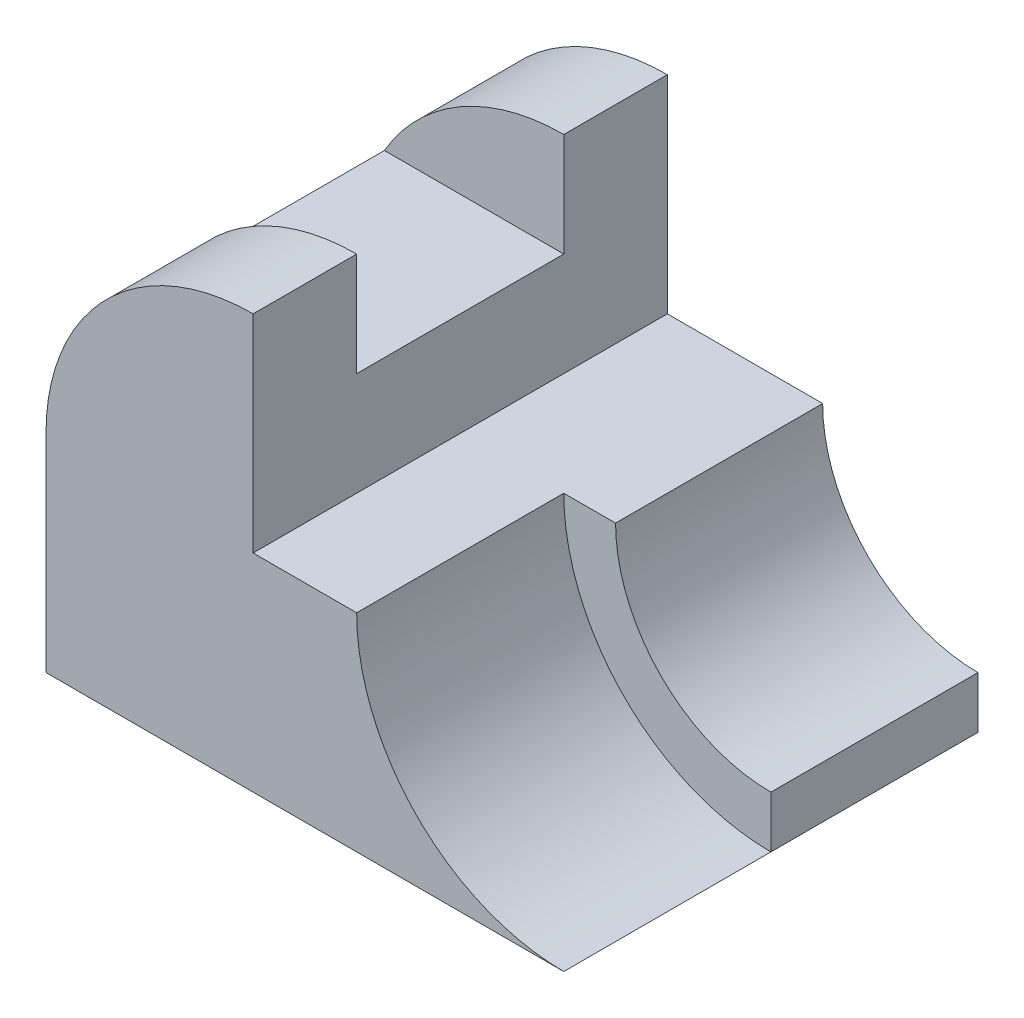
ISO-10303-21;
HEADER;
FILE_DESCRIPTION(('STEP AP214'),'2;1');
FILE_NAME('part.step','',(''),(''),'','','');
FILE_SCHEMA(('AUTOMOTIVE_DESIGN { 1 0 10303 214 1 1 1 1 }'));
ENDSEC;
DATA;
#1=APPLICATION_CONTEXT('core data for automotive mechanical design processes');
#2=APPLICATION_PROTOCOL_DEFINITION('international standard','automotive_design',2000,#1);
#3=PRODUCT_CONTEXT('',#1,'mechanical');
#4=PRODUCT('Part','Part','',(#3));
#5=PRODUCT_RELATED_PRODUCT_CATEGORY('part','',(#4));
#6=PRODUCT_DEFINITION_FORMATION('','',#4);
#7=PRODUCT_DEFINITION_CONTEXT('part definition',#1,'design');
#8=PRODUCT_DEFINITION('design','',#6,#7);
#9=PRODUCT_DEFINITION_SHAPE('','',#8);
#10=(LENGTH_UNIT() NAMED_UNIT(*) SI_UNIT(.MILLI.,.METRE.));
#11=(NAMED_UNIT(*) PLANE_ANGLE_UNIT() SI_UNIT($,.RADIAN.));
#12=(NAMED_UNIT(*) SI_UNIT($,.STERADIAN.) SOLID_ANGLE_UNIT());
#13=UNCERTAINTY_MEASURE_WITH_UNIT(LENGTH_MEASURE(1.E-05),#10,'distance_accuracy_value','');
#14=(GEOMETRIC_REPRESENTATION_CONTEXT(3) GLOBAL_UNCERTAINTY_ASSIGNED_CONTEXT((#13)) GLOBAL_UNIT_ASSIGNED_CONTEXT((#10,
#11,#12)) REPRESENTATION_CONTEXT('',''));
#15=CARTESIAN_POINT('',(0.,0.,0.));
#16=DIRECTION('',(0.,0.,1.));
#17=DIRECTION('',(1.,0.,0.));
#18=AXIS2_PLACEMENT_3D('',#15,#16,#17);
#19=CARTESIAN_POINT('',(50.,20.,-20.));
#20=DIRECTION('',(0.,-1.,0.));
#21=DIRECTION('',(1.,0.,0.));
#22=AXIS2_PLACEMENT_3D('',#19,#20,#21);
#23=PLANE('',#22);
#24=DIRECTION('',(1.,0.,0.));
#25=VECTOR('',#24,1.);
#26=CARTESIAN_POINT('',(50.,20.,-20.));
#27=LINE('',#26,#25);
#28=CARTESIAN_POINT('',(20.,20.,-20.));
#29=VERTEX_POINT('',#28);
#30=CARTESIAN_POINT('',(35.,20.,-20.));
#31=VERTEX_POINT('',#30);
#32=EDGE_CURVE('E173',#29,#31,#27,.T.);
#33=ORIENTED_EDGE('',*,*,#32,.F.);
#34=DIRECTION('',(0.,0.,1.));
#35=VECTOR('',#34,1.);
#36=CARTESIAN_POINT('',(20.,20.,-20.));
#37=LINE('',#36,#35);
#38=CARTESIAN_POINT('',(20.,20.,20.));
#39=VERTEX_POINT('',#38);
#40=EDGE_CURVE('E156',#29,#39,#37,.T.);
#41=ORIENTED_EDGE('',*,*,#40,.T.);
#42=DIRECTION('',(1.,0.,0.));
#43=VECTOR('',#42,1.);
#44=CARTESIAN_POINT('',(20.,20.,20.));
#45=LINE('',#44,#43);
#46=CARTESIAN_POINT('',(30.,20.,20.));
#47=VERTEX_POINT('',#46);
#48=EDGE_CURVE('E220',#39,#47,#45,.T.);
#49=ORIENTED_EDGE('',*,*,#48,.T.);
#50=DIRECTION('',(0.,0.,1.));
#51=VECTOR('',#50,1.);
#52=CARTESIAN_POINT('',(30.,20.,0.));
#53=LINE('',#52,#51);
#54=CARTESIAN_POINT('',(30.,20.,0.));
#55=VERTEX_POINT('',#54);
#56=EDGE_CURVE('E177',#55,#47,#53,.T.);
#57=ORIENTED_EDGE('',*,*,#56,.F.);
#58=DIRECTION('',(-1.,0.,0.));
#59=VECTOR('',#58,1.);
#60=CARTESIAN_POINT('',(30.,20.,0.));
#61=LINE('',#60,#59);
#62=CARTESIAN_POINT('',(35.,20.,0.));
#63=VERTEX_POINT('',#62);
#64=EDGE_CURVE('E185',#63,#55,#61,.T.);
#65=ORIENTED_EDGE('',*,*,#64,.F.);
#66=DIRECTION('',(0.,0.,1.));
#67=VECTOR('',#66,1.);
#68=CARTESIAN_POINT('',(35.,20.,-20.));
#69=LINE('',#68,#67);
#70=EDGE_CURVE('E53',#31,#63,#69,.T.);
#71=ORIENTED_EDGE('',*,*,#70,.F.);
#72=EDGE_LOOP('',(#33,#41,#49,#57,#65,#71));
#73=FACE_BOUND('',#72,.T.);
#74=ADVANCED_FACE('F39',(#73),#23,.F.);
#75=CARTESIAN_POINT('',(20.,43.4081818897871,9.99999999999999));
#76=DIRECTION('',(0.,0.,1.));
#77=DIRECTION('',(0.,-1.,0.));
#78=AXIS2_PLACEMENT_3D('',#75,#76,#77);
#79=PLANE('',#78);
#80=DIRECTION('',(1.,0.,0.));
#81=VECTOR('',#80,1.);
#82=CARTESIAN_POINT('',(19.9999999999999,30.,9.99999999999999));
#83=LINE('',#82,#81);
#84=CARTESIAN_POINT('',(2.67949192431127,30.,10.));
#85=VERTEX_POINT('',#84);
#86=CARTESIAN_POINT('',(19.9999999999999,30.,9.99999999999999));
#87=VERTEX_POINT('',#86);
#88=EDGE_CURVE('E147',#85,#87,#83,.T.);
#89=ORIENTED_EDGE('',*,*,#88,.F.);
#90=CARTESIAN_POINT('',(20.,19.9999999999999,10.));
#91=DIRECTION('',(0.,0.,1.));
#92=DIRECTION('',(0.,-1.,0.));
#93=AXIS2_PLACEMENT_3D('',#90,#91,#92);
#94=CIRCLE('',#93,20.);
#95=CARTESIAN_POINT('',(20.,40.,10.));
#96=VERTEX_POINT('',#95);
#97=EDGE_CURVE('E11',#96,#85,#94,.T.);
#98=ORIENTED_EDGE('',*,*,#97,.F.);
#99=DIRECTION('',(0.,1.,0.));
#100=VECTOR('',#99,1.);
#101=CARTESIAN_POINT('',(20.,43.4081818897871,9.99999999999999));
#102=LINE('',#101,#100);
#103=EDGE_CURVE('E214',#87,#96,#102,.T.);
#104=ORIENTED_EDGE('',*,*,#103,.F.);
#105=EDGE_LOOP('',(#89,#98,#104));
#106=FACE_BOUND('',#105,.T.);
#107=ADVANCED_FACE('F226',(#106),#79,.F.);
#108=CARTESIAN_POINT('',(20.,43.4081818897871,-10.));
#109=DIRECTION('',(0.,0.,-1.));
#110=DIRECTION('',(0.,1.,0.));
#111=AXIS2_PLACEMENT_3D('',#108,#109,#110);
#112=PLANE('',#111);
#113=DIRECTION('',(-1.,0.,0.));
#114=VECTOR('',#113,1.);
#115=CARTESIAN_POINT('',(0.,30.,-10.));
#116=LINE('',#115,#114);
#117=CARTESIAN_POINT('',(20.,30.,-10.));
#118=VERTEX_POINT('',#117);
#119=CARTESIAN_POINT('',(2.67949192431126,30.,-10.));
#120=VERTEX_POINT('',#119);
#121=EDGE_CURVE('E146',#118,#120,#116,.T.);
#122=ORIENTED_EDGE('',*,*,#121,.F.);
#123=DIRECTION('',(0.,-1.,0.));
#124=VECTOR('',#123,1.);
#125=CARTESIAN_POINT('',(20.,43.4081818897871,-10.));
#126=LINE('',#125,#124);
#127=CARTESIAN_POINT('',(20.,40.,-10.));
#128=VERTEX_POINT('',#127);
#129=EDGE_CURVE('E157',#128,#118,#126,.T.);
#130=ORIENTED_EDGE('',*,*,#129,.F.);
#131=CARTESIAN_POINT('',(20.,19.9999999999999,-10.));
#132=DIRECTION('',(0.,0.,-1.));
#133=DIRECTION('',(0.,1.,0.));
#134=AXIS2_PLACEMENT_3D('',#131,#132,#133);
#135=CIRCLE('',#134,20.);
#136=EDGE_CURVE('E50',#120,#128,#135,.T.);
#137=ORIENTED_EDGE('',*,*,#136,.F.);
#138=EDGE_LOOP('',(#122,#130,#137));
#139=FACE_BOUND('',#138,.T.);
#140=ADVANCED_FACE('F158',(#139),#112,.F.);
#141=CARTESIAN_POINT('',(50.,0.,20.));
#142=DIRECTION('',(-1.,0.,0.));
#143=DIRECTION('',(0.,-1.,0.));
#144=AXIS2_PLACEMENT_3D('',#141,#142,#143);
#145=PLANE('',#144);
#146=DIRECTION('',(0.,1.,0.));
#147=VECTOR('',#146,1.);
#148=CARTESIAN_POINT('',(50.,0.,-20.));
#149=LINE('',#148,#147);
#150=CARTESIAN_POINT('',(50.,0.,-20.));
#151=VERTEX_POINT('',#150);
#152=CARTESIAN_POINT('',(50.,5.,-20.));
#153=VERTEX_POINT('',#152);
#154=EDGE_CURVE('E168',#151,#153,#149,.T.);
#155=ORIENTED_EDGE('',*,*,#154,.T.);
#156=DIRECTION('',(0.,0.,1.));
#157=VECTOR('',#156,1.);
#158=CARTESIAN_POINT('',(50.,5.,-20.));
#159=LINE('',#158,#157);
#160=CARTESIAN_POINT('',(50.,5.,0.));
#161=VERTEX_POINT('',#160);
#162=EDGE_CURVE('E187',#153,#161,#159,.T.);
#163=ORIENTED_EDGE('',*,*,#162,.T.);
#164=DIRECTION('',(0.,1.,0.));
#165=VECTOR('',#164,1.);
#166=CARTESIAN_POINT('',(50.,0.,0.));
#167=LINE('',#166,#165);
#168=CARTESIAN_POINT('',(50.,0.,0.));
#169=VERTEX_POINT('',#168);
#170=EDGE_CURVE('E186',#169,#161,#167,.T.);
#171=ORIENTED_EDGE('',*,*,#170,.F.);
#172=DIRECTION('',(0.,0.,-1.));
#173=VECTOR('',#172,1.);
#174=CARTESIAN_POINT('',(50.,0.,20.));
#175=LINE('',#174,#173);
#176=EDGE_CURVE('E164',#169,#151,#175,.T.);
#177=ORIENTED_EDGE('',*,*,#176,.T.);
#178=EDGE_LOOP('',(#155,#163,#171,#177));
#179=FACE_BOUND('',#178,.T.);
#180=ADVANCED_FACE('F245',(#179),#145,.F.);
#181=CARTESIAN_POINT('',(0.,0.,20.));
#182=DIRECTION('',(1.,0.,0.));
#183=DIRECTION('',(0.,1.,0.));
#184=AXIS2_PLACEMENT_3D('',#181,#182,#183);
#185=PLANE('',#184);
#186=DIRECTION('',(0.,-1.,0.));
#187=VECTOR('',#186,1.);
#188=CARTESIAN_POINT('',(0.,0.,20.));
#189=LINE('',#188,#187);
#190=CARTESIAN_POINT('',(0.,20.,20.));
#191=VERTEX_POINT('',#190);
#192=CARTESIAN_POINT('',(0.,0.,20.));
#193=VERTEX_POINT('',#192);
#194=EDGE_CURVE('E64',#191,#193,#189,.T.);
#195=ORIENTED_EDGE('',*,*,#194,.F.);
#196=DIRECTION('',(0.,0.,1.));
#197=VECTOR('',#196,1.);
#198=CARTESIAN_POINT('',(0.,20.,-20.));
#199=LINE('',#198,#197);
#200=CARTESIAN_POINT('',(0.,20.,-20.));
#201=VERTEX_POINT('',#200);
#202=EDGE_CURVE('E198',#201,#191,#199,.T.);
#203=ORIENTED_EDGE('',*,*,#202,.F.);
#204=DIRECTION('',(0.,-1.,0.));
#205=VECTOR('',#204,1.);
#206=CARTESIAN_POINT('',(0.,0.,-20.));
#207=LINE('',#206,#205);
#208=CARTESIAN_POINT('',(0.,0.,-20.));
#209=VERTEX_POINT('',#208);
#210=EDGE_CURVE('E80',#201,#209,#207,.T.);
#211=ORIENTED_EDGE('',*,*,#210,.T.);
#212=DIRECTION('',(0.,0.,-1.));
#213=VECTOR('',#212,1.);
#214=CARTESIAN_POINT('',(0.,0.,20.));
#215=LINE('',#214,#213);
#216=EDGE_CURVE('E159',#193,#209,#215,.T.);
#217=ORIENTED_EDGE('',*,*,#216,.F.);
#218=EDGE_LOOP('',(#195,#203,#211,#217));
#219=FACE_BOUND('',#218,.T.);
#220=ADVANCED_FACE('F41',(#219),#185,.F.);
#221=CARTESIAN_POINT('',(0.,0.,20.));
#222=DIRECTION('',(0.,1.,0.));
#223=DIRECTION('',(0.,0.,1.));
#224=AXIS2_PLACEMENT_3D('',#221,#222,#223);
#225=PLANE('',#224);
#226=DIRECTION('',(1.,0.,0.));
#227=VECTOR('',#226,1.);
#228=CARTESIAN_POINT('',(0.,0.,-20.));
#229=LINE('',#228,#227);
#230=EDGE_CURVE('E169',#209,#151,#229,.T.);
#231=ORIENTED_EDGE('',*,*,#230,.T.);
#232=ORIENTED_EDGE('',*,*,#176,.F.);
#233=CARTESIAN_POINT('',(50.,0.,20.));
#234=VERTEX_POINT('',#233);
#235=EDGE_CURVE('E81',#234,#169,#175,.T.);
#236=ORIENTED_EDGE('',*,*,#235,.F.);
#237=DIRECTION('',(1.,0.,0.));
#238=VECTOR('',#237,1.);
#239=CARTESIAN_POINT('',(0.,0.,20.));
#240=LINE('',#239,#238);
#241=EDGE_CURVE('E172',#193,#234,#240,.T.);
#242=ORIENTED_EDGE('',*,*,#241,.F.);
#243=ORIENTED_EDGE('',*,*,#216,.T.);
#244=EDGE_LOOP('',(#231,#232,#236,#242,#243));
#245=FACE_BOUND('',#244,.T.);
#246=ADVANCED_FACE('F242',(#245),#225,.F.);
#247=CARTESIAN_POINT('',(0.,0.,20.));
#248=DIRECTION('',(0.,0.,-1.));
#249=DIRECTION('',(-1.,0.,0.));
#250=AXIS2_PLACEMENT_3D('',#247,#248,#249);
#251=PLANE('',#250);
#252=ORIENTED_EDGE('',*,*,#48,.F.);
#253=DIRECTION('',(0.,1.,0.));
#254=VECTOR('',#253,1.);
#255=CARTESIAN_POINT('',(20.,20.,20.));
#256=LINE('',#255,#254);
#257=CARTESIAN_POINT('',(20.,40.,20.));
#258=VERTEX_POINT('',#257);
#259=EDGE_CURVE('E213',#39,#258,#256,.T.);
#260=ORIENTED_EDGE('',*,*,#259,.T.);
#261=CARTESIAN_POINT('',(20.,19.9999999999999,20.));
#262=DIRECTION('',(0.,0.,-1.));
#263=DIRECTION('',(1.,0.,0.));
#264=AXIS2_PLACEMENT_3D('',#261,#262,#263);
#265=CIRCLE('',#264,20.);
#266=EDGE_CURVE('E207',#191,#258,#265,.T.);
#267=ORIENTED_EDGE('',*,*,#266,.F.);
#268=ORIENTED_EDGE('',*,*,#194,.T.);
#269=ORIENTED_EDGE('',*,*,#241,.T.);
#270=CARTESIAN_POINT('',(50.,20.,20.));
#271=DIRECTION('',(0.,0.,1.));
#272=DIRECTION('',(1.,0.,0.));
#273=AXIS2_PLACEMENT_3D('',#270,#271,#272);
#274=CIRCLE('',#273,20.);
#275=EDGE_CURVE('E182',#47,#234,#274,.T.);
#276=ORIENTED_EDGE('',*,*,#275,.F.);
#277=EDGE_LOOP('',(#252,#260,#267,#268,#269,#276));
#278=FACE_BOUND('',#277,.T.);
#279=ADVANCED_FACE('F233',(#278),#251,.F.);
#280=CARTESIAN_POINT('',(0.,0.,-20.));
#281=DIRECTION('',(0.,0.,-1.));
#282=DIRECTION('',(-1.,0.,0.));
#283=AXIS2_PLACEMENT_3D('',#280,#281,#282);
#284=PLANE('',#283);
#285=DIRECTION('',(0.,1.,0.));
#286=VECTOR('',#285,1.);
#287=CARTESIAN_POINT('',(20.,20.,-20.));
#288=LINE('',#287,#286);
#289=CARTESIAN_POINT('',(20.,40.,-20.));
#290=VERTEX_POINT('',#289);
#291=EDGE_CURVE('E219',#29,#290,#288,.T.);
#292=ORIENTED_EDGE('',*,*,#291,.F.);
#293=ORIENTED_EDGE('',*,*,#32,.T.);
#294=CARTESIAN_POINT('',(50.,20.,-20.));
#295=DIRECTION('',(0.,0.,1.));
#296=DIRECTION('',(1.,0.,0.));
#297=AXIS2_PLACEMENT_3D('',#294,#295,#296);
#298=CIRCLE('',#297,15.);
#299=EDGE_CURVE('E191',#31,#153,#298,.T.);
#300=ORIENTED_EDGE('',*,*,#299,.T.);
#301=ORIENTED_EDGE('',*,*,#154,.F.);
#302=ORIENTED_EDGE('',*,*,#230,.F.);
#303=ORIENTED_EDGE('',*,*,#210,.F.);
#304=CARTESIAN_POINT('',(20.,19.9999999999999,-20.));
#305=DIRECTION('',(0.,0.,-1.));
#306=DIRECTION('',(1.,0.,0.));
#307=AXIS2_PLACEMENT_3D('',#304,#305,#306);
#308=CIRCLE('',#307,20.);
#309=EDGE_CURVE('E209',#201,#290,#308,.T.);
#310=ORIENTED_EDGE('',*,*,#309,.T.);
#311=EDGE_LOOP('',(#292,#293,#300,#301,#302,#303,#310));
#312=FACE_BOUND('',#311,.T.);
#313=ADVANCED_FACE('F247',(#312),#284,.T.);
#314=CARTESIAN_POINT('',(50.,20.,0.));
#315=DIRECTION('',(0.,0.,1.));
#316=DIRECTION('',(1.,0.,0.));
#317=AXIS2_PLACEMENT_3D('',#314,#315,#316);
#318=CYLINDRICAL_SURFACE('',#317,20.);
#319=ORIENTED_EDGE('',*,*,#275,.T.);
#320=ORIENTED_EDGE('',*,*,#235,.T.);
#321=CARTESIAN_POINT('',(50.,20.,0.));
#322=DIRECTION('',(0.,0.,1.));
#323=DIRECTION('',(1.,0.,0.));
#324=AXIS2_PLACEMENT_3D('',#321,#322,#323);
#325=CIRCLE('',#324,20.);
#326=EDGE_CURVE('E184',#55,#169,#325,.T.);
#327=ORIENTED_EDGE('',*,*,#326,.F.);
#328=ORIENTED_EDGE('',*,*,#56,.T.);
#329=EDGE_LOOP('',(#319,#320,#327,#328));
#330=FACE_BOUND('',#329,.T.);
#331=ADVANCED_FACE('F236',(#330),#318,.F.);
#332=CARTESIAN_POINT('',(50.,20.,0.));
#333=DIRECTION('',(0.,0.,1.));
#334=DIRECTION('',(1.,0.,0.));
#335=AXIS2_PLACEMENT_3D('',#332,#333,#334);
#336=PLANE('',#335);
#337=CARTESIAN_POINT('',(50.,20.,0.));
#338=DIRECTION('',(0.,0.,1.));
#339=DIRECTION('',(1.,0.,0.));
#340=AXIS2_PLACEMENT_3D('',#337,#338,#339);
#341=CIRCLE('',#340,15.);
#342=EDGE_CURVE('E196',#63,#161,#341,.T.);
#343=ORIENTED_EDGE('',*,*,#342,.F.);
#344=ORIENTED_EDGE('',*,*,#64,.T.);
#345=ORIENTED_EDGE('',*,*,#326,.T.);
#346=ORIENTED_EDGE('',*,*,#170,.T.);
#347=EDGE_LOOP('',(#343,#344,#345,#346));
#348=FACE_BOUND('',#347,.T.);
#349=ADVANCED_FACE('F237',(#348),#336,.T.);
#350=CARTESIAN_POINT('',(50.,20.,-20.));
#351=DIRECTION('',(0.,0.,1.));
#352=DIRECTION('',(1.,0.,0.));
#353=AXIS2_PLACEMENT_3D('',#350,#351,#352);
#354=CYLINDRICAL_SURFACE('',#353,15.);
#355=ORIENTED_EDGE('',*,*,#342,.T.);
#356=ORIENTED_EDGE('',*,*,#162,.F.);
#357=ORIENTED_EDGE('',*,*,#299,.F.);
#358=ORIENTED_EDGE('',*,*,#70,.T.);
#359=EDGE_LOOP('',(#355,#356,#357,#358));
#360=FACE_BOUND('',#359,.T.);
#361=ADVANCED_FACE('F248',(#360),#354,.F.);
#362=CARTESIAN_POINT('',(20.,19.9999999999999,-20.));
#363=DIRECTION('',(0.,0.,1.));
#364=DIRECTION('',(1.,0.,0.));
#365=AXIS2_PLACEMENT_3D('',#362,#363,#364);
#366=CYLINDRICAL_SURFACE('',#365,20.);
#367=ORIENTED_EDGE('',*,*,#202,.T.);
#368=ORIENTED_EDGE('',*,*,#266,.T.);
#369=DIRECTION('',(0.,0.,1.));
#370=VECTOR('',#369,1.);
#371=CARTESIAN_POINT('',(20.,39.9999999999999,-20.));
#372=LINE('',#371,#370);
#373=EDGE_CURVE('E202',#96,#258,#372,.T.);
#374=ORIENTED_EDGE('',*,*,#373,.F.);
#375=ORIENTED_EDGE('',*,*,#97,.T.);
#376=DIRECTION('',(0.,0.,1.));
#377=VECTOR('',#376,1.);
#378=CARTESIAN_POINT('',(2.67949192431126,30.,-10.));
#379=LINE('',#378,#377);
#380=EDGE_CURVE('E136',#120,#85,#379,.T.);
#381=ORIENTED_EDGE('',*,*,#380,.F.);
#382=ORIENTED_EDGE('',*,*,#136,.T.);
#383=EDGE_CURVE('E205',#290,#128,#372,.T.);
#384=ORIENTED_EDGE('',*,*,#383,.F.);
#385=ORIENTED_EDGE('',*,*,#309,.F.);
#386=EDGE_LOOP('',(#367,#368,#374,#375,#381,#382,#384,#385));
#387=FACE_BOUND('',#386,.T.);
#388=ADVANCED_FACE('F138',(#387),#366,.T.);
#389=CARTESIAN_POINT('',(20.,20.,9.99999999999999));
#390=DIRECTION('',(-1.,0.,0.));
#391=DIRECTION('',(0.,0.,1.));
#392=AXIS2_PLACEMENT_3D('',#389,#390,#391);
#393=PLANE('',#392);
#394=ORIENTED_EDGE('',*,*,#373,.T.);
#395=ORIENTED_EDGE('',*,*,#259,.F.);
#396=ORIENTED_EDGE('',*,*,#40,.F.);
#397=ORIENTED_EDGE('',*,*,#291,.T.);
#398=ORIENTED_EDGE('',*,*,#383,.T.);
#399=ORIENTED_EDGE('',*,*,#129,.T.);
#400=DIRECTION('',(0.,0.,-1.));
#401=VECTOR('',#400,1.);
#402=CARTESIAN_POINT('',(20.,30.,-10.));
#403=LINE('',#402,#401);
#404=EDGE_CURVE('E151',#87,#118,#403,.T.);
#405=ORIENTED_EDGE('',*,*,#404,.F.);
#406=ORIENTED_EDGE('',*,*,#103,.T.);
#407=EDGE_LOOP('',(#394,#395,#396,#397,#398,#399,#405,#406));
#408=FACE_BOUND('',#407,.T.);
#409=ADVANCED_FACE('F227',(#408),#393,.F.);
#410=CARTESIAN_POINT('',(0.,30.,0.));
#411=DIRECTION('',(0.,-1.,0.));
#412=DIRECTION('',(1.,0.,0.));
#413=AXIS2_PLACEMENT_3D('',#410,#411,#412);
#414=PLANE('',#413);
#415=ORIENTED_EDGE('',*,*,#121,.T.);
#416=ORIENTED_EDGE('',*,*,#380,.T.);
#417=ORIENTED_EDGE('',*,*,#88,.T.);
#418=ORIENTED_EDGE('',*,*,#404,.T.);
#419=EDGE_LOOP('',(#415,#416,#417,#418));
#420=FACE_BOUND('',#419,.T.);
#421=ADVANCED_FACE('F148',(#420),#414,.F.);
#422=CLOSED_SHELL('',(#74,#107,#140,#180,#220,#246,#279,#313,#331,#349,#361,#388,#409,#421));
#423=MANIFOLD_SOLID_BREP('B2',#422);
#424=ADVANCED_BREP_SHAPE_REPRESENTATION('',(#18,#423),#14);
#425=SHAPE_DEFINITION_REPRESENTATION(#9,#424);
ENDSEC;
END-ISO-10303-21;
